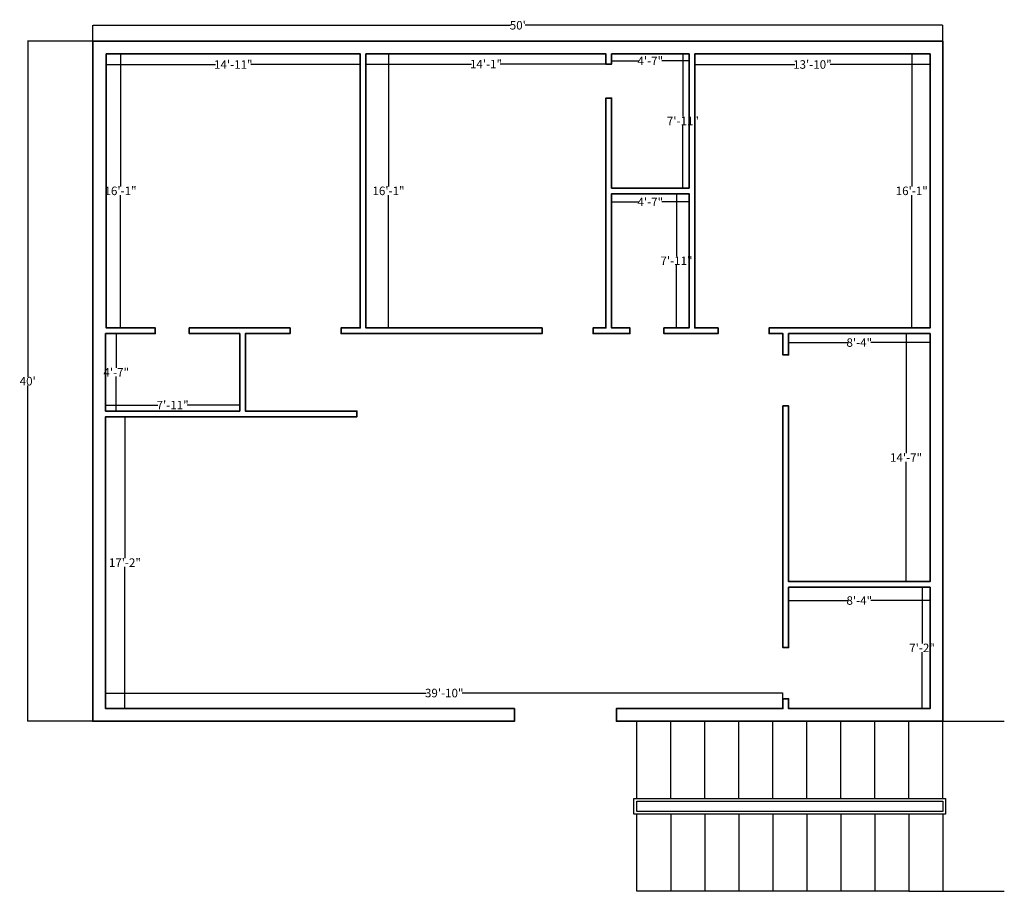
# Model space of a CAD drawing. Units: feet. Extents: x 3511 to 6270, y 2172 to 4127.
# Tile 2 of 4: x 4345 to 5040, y 3449 to 4064. Entities that reach past the tile are written whole.
import ezdxf

# ---------------------------------------------------------------- set-up
doc = ezdxf.new("R2010")
doc.units = ezdxf.units.FT
for name, color, linetype, lineweight in [('A-ANNO-DIMS', 2, 'Continuous', 18), ('A-FLOR-STRS', 4, 'Continuous', 25), ('A-WALL', 7, 'Continuous', 35)]:
    doc.layers.add(name, color=color, linetype=linetype, lineweight=lineweight)
doc.styles.get("Standard").update_dxf_attribs({"font": 'arial.ttf'})
doc.dimstyles.get("Standard").update_dxf_attribs({"dimtxt": 6, "dimasz": 0.18, "dimexe": 0.18, "dimexo": 0.0625, "dimgap": 0.09, "dimtad": 0, "dimtih": 1, "dimtoh": 1, "dimdec": 0, "dimzin": 0, "dimdsep": 46, "dimlunit": 3, "dimtxsty": 'Standard', "dimcen": 0.09, "dimadec": 0, "dimazin": 0, "dimtfac": 1, "dimtdec": 0, "dimtofl": 0, "dimtmove": 0, "dimatfit": 3, "dimfxl": 1, "dimtolj": 1, "dimtzin": 0, "dimarcsym": 0})

# ---------------------------------------------------------------- blocks, each defined once
blk = doc.blocks.new('*D32')
at = {"layer": 'A-ANNO-DIMS', "color": 0, "lineweight": -2, "transparency": 16777216}
for p, q in [((4405.77, 4039.51), (4405.77, 4031.86)), ((4585.11, 4039.51), (4585.11, 4031.86)), ((4405.95, 4032.04), (4483, 4032.04)), ((4584.93, 4032.04), (4507.88, 4032.04))]:
    blk.add_line(p, q, dxfattribs=at)
at = {"layer": 'A-ANNO-DIMS', "color": 0, "transparency": 16777216}
for points in [[(4405.95, 4032.07), (4405.95, 4032.01), (4405.77, 4032.04)], [(4584.93, 4032.07), (4584.93, 4032.01), (4585.11, 4032.04)]]:
    blk.add_solid(points, dxfattribs=at)
at = {"layer": 'Defpoints', "color": 0, "transparency": 16777216}
for p in [(4405.77, 4039.58), (4585.11, 4039.58), (4585.11, 4032.04)]:
    blk.add_point(p, dxfattribs=at)
at = {"layer": 'A-ANNO-DIMS', "color": 0, "transparency": 16777216, "insert": (4495.44, 4032.04), "char_height": 6, "attachment_point": 5}
blk.add_mtext('\\A1;14\'-11"', dxfattribs=at)
blk = doc.blocks.new('*D23')
at = {"layer": 'A-ANNO-DIMS', "color": 0, "lineweight": -2, "transparency": 16777216}
for p, q in [((4405.83, 4039.58), (4416.04, 4039.58)), ((4415.86, 4039.4), (4415.86, 3946.05)), ((4415.86, 3846.39), (4415.86, 3939.74)), ((4405.83, 3846.21), (4416.04, 3846.21))]:
    blk.add_line(p, q, dxfattribs=at)
at = {"layer": 'A-ANNO-DIMS', "color": 0, "transparency": 16777216}
for points in [[(4415.83, 4039.4), (4415.89, 4039.4), (4415.86, 4039.58)], [(4415.83, 3846.39), (4415.89, 3846.39), (4415.86, 3846.21)]]:
    blk.add_solid(points, dxfattribs=at)
at = {"layer": 'Defpoints', "color": 0, "transparency": 16777216}
for p in [(4405.77, 4039.58), (4405.77, 3846.21), (4415.86, 3846.21)]:
    blk.add_point(p, dxfattribs=at)
at = {"layer": 'A-ANNO-DIMS', "color": 0, "transparency": 16777216, "insert": (4415.86, 3942.89), "char_height": 6, "attachment_point": 5}
blk.add_mtext('\\A1;16\'-1"', dxfattribs=at)
blk = doc.blocks.new('*D24')
at = {"layer": 'A-ANNO-DIMS', "color": 0, "lineweight": -2, "transparency": 16777216}
for p, q in [((4589.11, 4039.51), (4589.11, 4032.14)), ((4758.44, 4039.51), (4758.44, 4032.14)), ((4589.29, 4032.32), (4663.66, 4032.32)), ((4758.26, 4032.32), (4683.89, 4032.32))]:
    blk.add_line(p, q, dxfattribs=at)
at = {"layer": 'A-ANNO-DIMS', "color": 0, "transparency": 16777216}
for points in [[(4589.29, 4032.35), (4589.29, 4032.29), (4589.11, 4032.32)], [(4758.26, 4032.35), (4758.26, 4032.29), (4758.44, 4032.32)]]:
    blk.add_solid(points, dxfattribs=at)
at = {"layer": 'Defpoints', "color": 0, "transparency": 16777216}
for p in [(4589.11, 4039.58), (4758.44, 4039.58), (4758.44, 4032.32)]:
    blk.add_point(p, dxfattribs=at)
at = {"layer": 'A-ANNO-DIMS', "color": 0, "transparency": 16777216, "insert": (4673.78, 4032.32), "char_height": 6, "attachment_point": 5}
blk.add_mtext('\\A1;14\'-1"', dxfattribs=at)
blk = doc.blocks.new('*D25')
at = {"layer": 'A-ANNO-DIMS', "color": 0, "lineweight": -2, "transparency": 16777216}
for p, q in [((4589.17, 4039.58), (4605.2, 4039.58)), ((4605.02, 4039.4), (4605.02, 3946.05)), ((4605.02, 3846.39), (4605.02, 3939.74)), ((4589.17, 3846.21), (4605.2, 3846.21))]:
    blk.add_line(p, q, dxfattribs=at)
at = {"layer": 'A-ANNO-DIMS', "color": 0, "transparency": 16777216}
for points in [[(4604.99, 4039.4), (4605.05, 4039.4), (4605.02, 4039.58)], [(4604.99, 3846.39), (4605.05, 3846.39), (4605.02, 3846.21)]]:
    blk.add_solid(points, dxfattribs=at)
at = {"layer": 'Defpoints', "color": 0, "transparency": 16777216}
for p in [(4589.11, 4039.58), (4589.11, 3846.21), (4605.02, 3846.21)]:
    blk.add_point(p, dxfattribs=at)
at = {"layer": 'A-ANNO-DIMS', "color": 0, "transparency": 16777216, "insert": (4605.02, 3942.89), "char_height": 6, "attachment_point": 5}
blk.add_mtext('\\A1;16\'-1"', dxfattribs=at)
blk = doc.blocks.new('*D26')
at = {"layer": 'A-ANNO-DIMS', "color": 0, "lineweight": -2, "transparency": 16777216}
for p, q in [((4762.44, 4039.51), (4762.44, 4034.45)), ((4817.15, 4039.51), (4817.15, 4034.45)), ((4762.62, 4034.63), (4781.61, 4034.63)), ((4816.97, 4034.63), (4797.98, 4034.63))]:
    blk.add_line(p, q, dxfattribs=at)
at = {"layer": 'A-ANNO-DIMS', "color": 0, "transparency": 16777216}
for points in [[(4762.62, 4034.66), (4762.62, 4034.6), (4762.44, 4034.63)], [(4816.97, 4034.66), (4816.97, 4034.6), (4817.15, 4034.63)]]:
    blk.add_solid(points, dxfattribs=at)
at = {"layer": 'Defpoints', "color": 0, "transparency": 16777216}
for p in [(4762.44, 4039.58), (4817.15, 4039.58), (4817.15, 4034.63)]:
    blk.add_point(p, dxfattribs=at)
at = {"layer": 'A-ANNO-DIMS', "color": 0, "transparency": 16777216, "insert": (4789.8, 4034.63), "char_height": 6, "attachment_point": 5}
blk.add_mtext('\\A1;4\'-7"', dxfattribs=at)
blk = doc.blocks.new('*D27')
at = {"layer": 'A-ANNO-DIMS', "color": 0, "lineweight": -2, "transparency": 16777216}
for p, q in [((4817.09, 4039.58), (4812.63, 4039.58)), ((4812.81, 4039.4), (4812.81, 3995.34)), ((4812.81, 3945.07), (4812.81, 3989.13)), ((4817.09, 3944.89), (4812.63, 3944.89))]:
    blk.add_line(p, q, dxfattribs=at)
at = {"layer": 'A-ANNO-DIMS', "color": 0, "transparency": 16777216}
for points in [[(4812.78, 4039.4), (4812.84, 4039.4), (4812.81, 4039.58)], [(4812.78, 3945.07), (4812.84, 3945.07), (4812.81, 3944.89)]]:
    blk.add_solid(points, dxfattribs=at)
at = {"layer": 'Defpoints', "color": 0, "transparency": 16777216}
for p in [(4817.15, 4039.58), (4812.81, 3944.89), (4817.15, 3944.89)]:
    blk.add_point(p, dxfattribs=at)
at = {"layer": 'A-ANNO-DIMS', "color": 0, "transparency": 16777216, "insert": (4812.81, 3992.23), "char_height": 6, "attachment_point": 5}
blk.add_mtext('\\A1;7\'-11"', dxfattribs=at)
blk = doc.blocks.new('*D28')
at = {"layer": 'A-ANNO-DIMS', "color": 0, "lineweight": -2, "transparency": 16777216}
for p, q in [((4821.15, 4039.51), (4821.15, 4031.89)), ((4987.28, 4039.51), (4987.28, 4031.89)), ((4821.33, 4032.07), (4891.77, 4032.07)), ((4987.1, 4032.07), (4916.66, 4032.07))]:
    blk.add_line(p, q, dxfattribs=at)
at = {"layer": 'A-ANNO-DIMS', "color": 0, "transparency": 16777216}
for points in [[(4821.33, 4032.1), (4821.33, 4032.04), (4821.15, 4032.07)], [(4987.1, 4032.1), (4987.1, 4032.04), (4987.28, 4032.07)]]:
    blk.add_solid(points, dxfattribs=at)
at = {"layer": 'Defpoints', "color": 0, "transparency": 16777216}
for p in [(4821.15, 4039.58), (4987.28, 4039.58), (4987.28, 4032.07)]:
    blk.add_point(p, dxfattribs=at)
at = {"layer": 'A-ANNO-DIMS', "color": 0, "transparency": 16777216, "insert": (4904.22, 4032.07), "char_height": 6, "attachment_point": 5}
blk.add_mtext('\\A1;13\'-10"', dxfattribs=at)
blk = doc.blocks.new('*D29')
at = {"layer": 'A-ANNO-DIMS', "color": 0, "lineweight": -2, "transparency": 16777216}
for p, q in [((4987.22, 4039.58), (4974.16, 4039.58)), ((4974.34, 4039.4), (4974.34, 3946.05)), ((4974.34, 3846.39), (4974.34, 3939.74)), ((4987.22, 3846.21), (4974.16, 3846.21))]:
    blk.add_line(p, q, dxfattribs=at)
at = {"layer": 'A-ANNO-DIMS', "color": 0, "transparency": 16777216}
for points in [[(4974.31, 4039.4), (4974.37, 4039.4), (4974.34, 4039.58)], [(4974.31, 3846.39), (4974.37, 3846.39), (4974.34, 3846.21)]]:
    blk.add_solid(points, dxfattribs=at)
at = {"layer": 'Defpoints', "color": 0, "transparency": 16777216}
for p in [(4987.28, 4039.58), (4974.34, 3846.21), (4987.28, 3846.21)]:
    blk.add_point(p, dxfattribs=at)
at = {"layer": 'A-ANNO-DIMS', "color": 0, "transparency": 16777216, "insert": (4974.34, 3942.89), "char_height": 6, "attachment_point": 5}
blk.add_mtext('\\A1;16\'-1"', dxfattribs=at)
blk = doc.blocks.new('*D30')
at = {"layer": 'A-ANNO-DIMS', "color": 0, "lineweight": -2, "transparency": 16777216}
for p, q in [((4817.09, 3940.89), (4808.08, 3940.89)), ((4808.26, 3940.71), (4808.26, 3896.65)), ((4808.26, 3846.39), (4808.26, 3890.45)), ((4817.09, 3846.21), (4808.08, 3846.21))]:
    blk.add_line(p, q, dxfattribs=at)
at = {"layer": 'A-ANNO-DIMS', "color": 0, "transparency": 16777216}
for points in [[(4808.23, 3940.71), (4808.29, 3940.71), (4808.26, 3940.89)], [(4808.23, 3846.39), (4808.29, 3846.39), (4808.26, 3846.21)]]:
    blk.add_solid(points, dxfattribs=at)
at = {"layer": 'Defpoints', "color": 0, "transparency": 16777216}
for p in [(4817.15, 3940.89), (4808.26, 3846.21), (4817.15, 3846.21)]:
    blk.add_point(p, dxfattribs=at)
at = {"layer": 'A-ANNO-DIMS', "color": 0, "transparency": 16777216, "insert": (4808.26, 3893.55), "char_height": 6, "attachment_point": 5}
blk.add_mtext('\\A1;7\'-11"', dxfattribs=at)
blk = doc.blocks.new('*D31')
at = {"layer": 'A-ANNO-DIMS', "color": 0, "lineweight": -2, "transparency": 16777216}
for p, q in [((4762.44, 3940.83), (4762.44, 3934.92)), ((4817.15, 3940.83), (4817.15, 3934.92)), ((4762.62, 3935.1), (4781.61, 3935.1)), ((4816.97, 3935.1), (4797.98, 3935.1))]:
    blk.add_line(p, q, dxfattribs=at)
at = {"layer": 'A-ANNO-DIMS', "color": 0, "transparency": 16777216}
for points in [[(4762.62, 3935.13), (4762.62, 3935.07), (4762.44, 3935.1)], [(4816.97, 3935.13), (4816.97, 3935.07), (4817.15, 3935.1)]]:
    blk.add_solid(points, dxfattribs=at)
at = {"layer": 'Defpoints', "color": 0, "transparency": 16777216}
for p in [(4762.44, 3940.89), (4817.15, 3940.89), (4817.15, 3935.1)]:
    blk.add_point(p, dxfattribs=at)
at = {"layer": 'A-ANNO-DIMS', "color": 0, "transparency": 16777216, "insert": (4789.8, 3935.1), "char_height": 6, "attachment_point": 5}
blk.add_mtext('\\A1;4\'-7"', dxfattribs=at)
blk = doc.blocks.new('*D33')
at = {"layer": 'A-ANNO-DIMS', "color": 0, "lineweight": -2, "transparency": 16777216}
for p, q in [((4405.28, 3787.57), (4405.28, 3791.87)), ((4405.46, 3791.69), (4442.25, 3791.69)), ((4499.79, 3791.69), (4462.99, 3791.69)), ((4499.97, 3787.57), (4499.97, 3791.87))]:
    blk.add_line(p, q, dxfattribs=at)
at = {"layer": 'A-ANNO-DIMS', "color": 0, "transparency": 16777216}
for points in [[(4405.46, 3791.72), (4405.46, 3791.66), (4405.28, 3791.69)], [(4499.79, 3791.72), (4499.79, 3791.66), (4499.97, 3791.69)]]:
    blk.add_solid(points, dxfattribs=at)
at = {"layer": 'Defpoints', "color": 0, "transparency": 16777216}
for p in [(4499.97, 3791.69), (4405.28, 3787.5), (4499.97, 3787.5)]:
    blk.add_point(p, dxfattribs=at)
at = {"layer": 'A-ANNO-DIMS', "color": 0, "transparency": 16777216, "insert": (4452.62, 3791.69), "char_height": 6, "attachment_point": 5}
blk.add_mtext('\\A1;7\'-11"', dxfattribs=at)
blk = doc.blocks.new('*D34')
at = {"layer": 'A-ANNO-DIMS', "color": 0, "lineweight": -2, "transparency": 16777216}
for p, q in [((4405.34, 3842.21), (4412.98, 3842.21)), ((4412.8, 3842.03), (4412.8, 3817.95)), ((4412.8, 3787.68), (4412.8, 3811.77)), ((4405.34, 3787.5), (4412.98, 3787.5))]:
    blk.add_line(p, q, dxfattribs=at)
at = {"layer": 'A-ANNO-DIMS', "color": 0, "transparency": 16777216}
for points in [[(4412.77, 3842.03), (4412.83, 3842.03), (4412.8, 3842.21)], [(4412.77, 3787.68), (4412.83, 3787.68), (4412.8, 3787.5)]]:
    blk.add_solid(points, dxfattribs=at)
at = {"layer": 'Defpoints', "color": 0, "transparency": 16777216}
for p in [(4405.28, 3842.21), (4412.8, 3842.21), (4405.28, 3787.5)]:
    blk.add_point(p, dxfattribs=at)
at = {"layer": 'A-ANNO-DIMS', "color": 0, "transparency": 16777216, "insert": (4412.8, 3814.86), "char_height": 6, "attachment_point": 5}
blk.add_mtext('\\A1;4\'-7"', dxfattribs=at)
blk = doc.blocks.new('*D35')
at = {"layer": 'A-ANNO-DIMS', "color": 0, "lineweight": -2, "transparency": 16777216}
for p, q in [((4405.28, 3577.64), (4405.28, 3588.67)), ((4405.46, 3588.49), (4631.6, 3588.49)), ((4883.19, 3588.49), (4657.05, 3588.49)), ((4883.37, 3577.64), (4883.37, 3588.67))]:
    blk.add_line(p, q, dxfattribs=at)
at = {"layer": 'A-ANNO-DIMS', "color": 0, "transparency": 16777216}
for points in [[(4405.46, 3588.52), (4405.46, 3588.46), (4405.28, 3588.49)], [(4883.19, 3588.52), (4883.19, 3588.46), (4883.37, 3588.49)]]:
    blk.add_solid(points, dxfattribs=at)
at = {"layer": 'Defpoints', "color": 0, "transparency": 16777216}
for p in [(4883.37, 3588.49), (4405.28, 3577.58), (4883.37, 3577.58)]:
    blk.add_point(p, dxfattribs=at)
at = {"layer": 'A-ANNO-DIMS', "color": 0, "transparency": 16777216, "insert": (4644.33, 3588.49), "char_height": 6, "attachment_point": 5}
blk.add_mtext('\\A1;39\'-10"', dxfattribs=at)
blk = doc.blocks.new('*D36')
at = {"layer": 'A-ANNO-DIMS', "color": 0, "lineweight": -2, "transparency": 16777216}
for p, q in [((4405.34, 3783.5), (4419.1, 3783.5)), ((4418.92, 3783.32), (4418.92, 3683.64)), ((4418.92, 3577.76), (4418.92, 3677.44)), ((4405.34, 3577.58), (4419.1, 3577.58))]:
    blk.add_line(p, q, dxfattribs=at)
at = {"layer": 'A-ANNO-DIMS', "color": 0, "transparency": 16777216}
for points in [[(4418.89, 3783.32), (4418.95, 3783.32), (4418.92, 3783.5)], [(4418.89, 3577.76), (4418.95, 3577.76), (4418.92, 3577.58)]]:
    blk.add_solid(points, dxfattribs=at)
at = {"layer": 'Defpoints', "color": 0, "transparency": 16777216}
for p in [(4405.28, 3783.5), (4405.28, 3577.58), (4418.92, 3577.58)]:
    blk.add_point(p, dxfattribs=at)
at = {"layer": 'A-ANNO-DIMS', "color": 0, "transparency": 16777216, "insert": (4418.92, 3680.54), "char_height": 6, "attachment_point": 5}
blk.add_mtext('\\A1;17\'-2"', dxfattribs=at)
blk = doc.blocks.new('*D37')
at = {"layer": 'A-ANNO-DIMS', "color": 0, "lineweight": -2, "transparency": 16777216}
for p, q in [((4987.22, 3842.21), (4970.13, 3842.21)), ((4970.31, 3842.03), (4970.31, 3757.78)), ((4970.31, 3667.33), (4970.31, 3751.57)), ((4987.22, 3667.15), (4970.13, 3667.15))]:
    blk.add_line(p, q, dxfattribs=at)
at = {"layer": 'A-ANNO-DIMS', "color": 0, "transparency": 16777216}
for points in [[(4970.28, 3842.03), (4970.34, 3842.03), (4970.31, 3842.21)], [(4970.28, 3667.33), (4970.34, 3667.33), (4970.31, 3667.15)]]:
    blk.add_solid(points, dxfattribs=at)
at = {"layer": 'Defpoints', "color": 0, "transparency": 16777216}
for p in [(4987.28, 3842.21), (4970.31, 3667.15), (4987.28, 3667.15)]:
    blk.add_point(p, dxfattribs=at)
at = {"layer": 'A-ANNO-DIMS', "color": 0, "transparency": 16777216, "insert": (4970.31, 3754.68), "char_height": 6, "attachment_point": 5}
blk.add_mtext('\\A1;14\'-7"', dxfattribs=at)
blk = doc.blocks.new('*D38')
at = {"layer": 'A-ANNO-DIMS', "color": 0, "lineweight": -2, "transparency": 16777216}
for p, q in [((4887.37, 3842.15), (4887.37, 3835.65)), ((4987.28, 3842.15), (4987.28, 3835.65)), ((4887.55, 3835.83), (4929.26, 3835.83)), ((4987.1, 3835.83), (4945.39, 3835.83))]:
    blk.add_line(p, q, dxfattribs=at)
at = {"layer": 'A-ANNO-DIMS', "color": 0, "transparency": 16777216}
for points in [[(4887.55, 3835.86), (4887.55, 3835.8), (4887.37, 3835.83)], [(4987.1, 3835.86), (4987.1, 3835.8), (4987.28, 3835.83)]]:
    blk.add_solid(points, dxfattribs=at)
at = {"layer": 'Defpoints', "color": 0, "transparency": 16777216}
for p in [(4887.37, 3842.21), (4987.28, 3842.21), (4887.37, 3835.83)]:
    blk.add_point(p, dxfattribs=at)
at = {"layer": 'A-ANNO-DIMS', "color": 0, "transparency": 16777216, "insert": (4937.33, 3835.83), "char_height": 6, "attachment_point": 5}
blk.add_mtext('\\A1;8\'-4"', dxfattribs=at)
blk = doc.blocks.new('*D39')
at = {"layer": 'A-ANNO-DIMS', "color": 0, "lineweight": -2, "transparency": 16777216}
for p, q in [((4987.22, 3663.15), (4981.44, 3663.15)), ((4981.62, 3662.97), (4981.62, 3623.46)), ((4981.62, 3577.76), (4981.62, 3617.26)), ((4987.22, 3577.58), (4981.44, 3577.58))]:
    blk.add_line(p, q, dxfattribs=at)
at = {"layer": 'A-ANNO-DIMS', "color": 0, "transparency": 16777216}
for points in [[(4981.59, 3662.97), (4981.65, 3662.97), (4981.62, 3663.15)], [(4981.59, 3577.76), (4981.65, 3577.76), (4981.62, 3577.58)]]:
    blk.add_solid(points, dxfattribs=at)
at = {"layer": 'Defpoints', "color": 0, "transparency": 16777216}
for p in [(4987.28, 3663.15), (4981.62, 3577.58), (4987.28, 3577.58)]:
    blk.add_point(p, dxfattribs=at)
at = {"layer": 'A-ANNO-DIMS', "color": 0, "transparency": 16777216, "insert": (4981.62, 3620.36), "char_height": 6, "attachment_point": 5}
blk.add_mtext('\\A1;7\'-2"', dxfattribs=at)
blk = doc.blocks.new('*D40')
at = {"layer": 'A-ANNO-DIMS', "color": 0, "lineweight": -2, "transparency": 16777216}
for p, q in [((4887.37, 3663.08), (4887.37, 3653.6)), ((4987.28, 3663.08), (4987.28, 3653.6)), ((4887.55, 3653.78), (4929.26, 3653.78)), ((4987.1, 3653.78), (4945.39, 3653.78))]:
    blk.add_line(p, q, dxfattribs=at)
at = {"layer": 'A-ANNO-DIMS', "color": 0, "transparency": 16777216}
for points in [[(4887.55, 3653.81), (4887.55, 3653.75), (4887.37, 3653.78)], [(4987.1, 3653.81), (4987.1, 3653.75), (4987.28, 3653.78)]]:
    blk.add_solid(points, dxfattribs=at)
at = {"layer": 'Defpoints', "color": 0, "transparency": 16777216}
for p in [(4887.37, 3663.15), (4987.28, 3663.15), (4887.37, 3653.78)]:
    blk.add_point(p, dxfattribs=at)
at = {"layer": 'A-ANNO-DIMS', "color": 0, "transparency": 16777216, "insert": (4937.33, 3653.78), "char_height": 6, "attachment_point": 5}
blk.add_mtext('\\A1;8\'-4"', dxfattribs=at)
blk = doc.blocks.new('*D41')
at = {"layer": 'A-ANNO-DIMS', "color": 0, "lineweight": -2, "transparency": 16777216}
for p, q in [((4396.22, 4048.58), (4350.17, 4048.58)), ((4350.35, 4048.4), (4350.35, 3811.73)), ((4350.35, 3568.76), (4350.35, 3805.42)), ((4396.22, 3568.58), (4350.17, 3568.58))]:
    blk.add_line(p, q, dxfattribs=at)
at = {"layer": 'A-ANNO-DIMS', "color": 0, "transparency": 16777216}
for points in [[(4350.32, 4048.4), (4350.38, 4048.4), (4350.35, 4048.58)], [(4350.32, 3568.76), (4350.38, 3568.76), (4350.35, 3568.58)]]:
    blk.add_solid(points, dxfattribs=at)
at = {"layer": 'Defpoints', "color": 0, "transparency": 16777216}
for p in [(4396.28, 4048.58), (4350.35, 3568.58), (4396.28, 3568.58)]:
    blk.add_point(p, dxfattribs=at)
at = {"layer": 'A-ANNO-DIMS', "color": 0, "transparency": 16777216, "insert": (4350.35, 3808.58), "char_height": 6, "attachment_point": 5}
blk.add_mtext("\\A1;40'", dxfattribs=at)
blk = doc.blocks.new('*D42')
at = {"layer": 'A-ANNO-DIMS', "color": 0, "lineweight": -2, "transparency": 16777216}
for p, q in [((4396.28, 4048.64), (4396.28, 4059.92)), ((4396.46, 4059.74), (4691.1, 4059.74)), ((4996.1, 4059.74), (4701.46, 4059.74)), ((4996.28, 4048.64), (4996.28, 4059.92))]:
    blk.add_line(p, q, dxfattribs=at)
at = {"layer": 'A-ANNO-DIMS', "color": 0, "transparency": 16777216}
for points in [[(4396.46, 4059.77), (4396.46, 4059.71), (4396.28, 4059.74)], [(4996.1, 4059.77), (4996.1, 4059.71), (4996.28, 4059.74)]]:
    blk.add_solid(points, dxfattribs=at)
at = {"layer": 'Defpoints', "color": 0, "transparency": 16777216}
for p in [(4996.28, 4059.74), (4396.28, 4048.58), (4996.28, 4048.58)]:
    blk.add_point(p, dxfattribs=at)
at = {"layer": 'A-ANNO-DIMS', "color": 0, "transparency": 16777216, "insert": (4696.28, 4059.74), "char_height": 6, "attachment_point": 5}
blk.add_mtext("\\A1;50'", dxfattribs=at)
blk = doc.blocks.new('STAIR')
for p, q in [((2, 65.57), (2, 120)), ((26, 65.57), (26, 120)), ((50, 65.57), (50, 120)), ((74, 65.57), (74, 120)), ((98, 65.57), (98, 120)), ((122, 65.57), (122, 120)), ((146, 65.57), (146, 120)), ((170, 65.57), (170, 120)), ((194, 65.57), (194, 120)), ((218, 54.42), (218, 0))]:
    blk.add_line(p, q)
for points in [[(218, 65.57), (218, 120), (261.4, 120)], [(26, 54.42), (26, 0), (14, 0), (2, 0), (2, 54.42)], [(50, 54.42), (50, 0), (38, 0), (26, 0)], [(74, 54.42), (74, 0), (62, 0), (50, 0)], [(98, 54.42), (98, 0), (86, 0), (74, 0)], [(122, 54.42), (122, 0), (110, 0), (98, 0)], [(146, 54.42), (146, 0), (134, 0), (122, 0)], [(170, 54.42), (170, 0), (158, 0), (146, 0)], [(194, 54.42), (194, 0), (182, 0), (170, 0)], [(194, 0), (206, 0), (218, 0), (261.4, 0)]]:
    blk.add_lwpolyline(points)
for points in [[(0, 65.57), (220, 65.57), (220, 54.42), (0, 54.42)], [(218, 56.42), (2, 56.42), (2, 63.57), (218, 63.57)]]:
    blk.add_lwpolyline(points, close=True)

msp = doc.modelspace()

# ---------------------------------------------------------------- linework, layer by layer
at = {"layer": 'A-WALL'}
msp.add_lwpolyline([(4887.37, 3663.15), (4887.37, 3620.52), (4883.37, 3620.52), (4883.37, 3791.14), (4887.37, 3791.14), (4887.37, 3667.15), (4987.28, 3667.15), (4987.28, 3842.21), (4887.37, 3842.21), (4887.37, 3827.14), (4883.37, 3827.14), (4883.37, 3842.21), (4873.69, 3842.21), (4873.69, 3846.21), (4987.28, 3846.21), (4987.28, 4039.58), (4821.15, 4039.58), (4821.15, 3846.21), (4837.69, 3846.21), (4837.69, 3842.21), (4799.38, 3842.21), (4799.38, 3846.21), (4817.15, 3846.21), (4817.15, 3940.89), (4762.44, 3940.89), (4762.44, 3846.21), (4775.38, 3846.21), (4775.38, 3842.21), (4749.44, 3842.21), (4749.44, 3846.21), (4758.44, 3846.21), (4758.44, 4008.32), (4762.44, 4008.32), (4762.44, 3944.89), (4817.15, 3944.89), (4817.15, 4039.58), (4762.44, 4039.58), (4762.44, 4032.32), (4758.44, 4032.32), (4758.44, 4039.58), (4589.11, 4039.58), (4589.11, 3846.21), (4713.44, 3846.21), (4713.44, 3842.21), (4571.55, 3842.21), (4571.55, 3846.21), (4585.11, 3846.21), (4585.11, 4039.58), (4405.77, 4039.58), (4405.77, 3846.21), (4440.3, 3846.21), (4440.3, 3842.21), (4405.28, 3842.21), (4405.28, 3787.5), (4405.28, 3787.5), (4499.97, 3787.5), (4499.97, 3842.21), (4464.3, 3842.21), (4464.3, 3846.21), (4535.55, 3846.21), (4535.55, 3842.21), (4503.97, 3842.21), (4503.97, 3787.51), (4582.72, 3787.51), (4582.72, 3783.5), (4405.28, 3783.5), (4405.28, 3577.58), (4693.92, 3577.58), (4693.92, 3568.58), (4396.28, 3568.58), (4396.28, 4048.58), (4996.28, 4048.58), (4996.28, 3568.58), (4765.92, 3568.58), (4765.92, 3577.58), (4883.37, 3577.58), (4883.37, 3584.52), (4887.37, 3584.52), (4887.37, 3577.58), (4987.28, 3577.58), (4987.28, 3663.15)], close=True, dxfattribs=at)
msp.add_lwpolyline([(4503.97, 3783.5), (4503.97, 3783.5)], dxfattribs=at)

# ---------------------------------------------------------------- block references
at = {"layer": 'A-FLOR-STRS'}
msp.add_blockref('STAIR', (4778.28, 3448.58), dxfattribs=at)

# ---------------------------------------------------------------- dimensions: what is measured, and where the dimension line sits
at = {"layer": 'A-ANNO-DIMS'}
for base, p1, p2, picture, middle in [((4996.28, 4059.74), (4396.28, 4048.58), (4996.28, 4048.58), '*D42', (4696.28, 4059.74)), ((4585.11, 4032.04), (4405.77, 4039.58), (4585.11, 4039.58), '*D32', (4495.44, 4032.04)), ((4758.44, 4032.32), (4589.11, 4039.58), (4758.44, 4039.58), '*D24', (4673.78, 4032.32)), ((4817.15, 4034.63), (4762.44, 4039.58), (4817.15, 4039.58), '*D26', (4789.8, 4034.63)), ((4987.28, 4032.07), (4821.15, 4039.58), (4987.28, 4039.58), '*D28', (4904.22, 4032.07)), ((4817.15, 3935.1), (4762.44, 3940.89), (4817.15, 3940.89), '*D31', (4789.8, 3935.1)), ((4887.37, 3835.83), (4987.28, 3842.21), (4887.37, 3842.21), '*D38', (4937.33, 3835.83)), ((4499.97, 3791.69), (4405.28, 3787.5), (4499.97, 3787.5), '*D33', (4452.62, 3791.69)), ((4887.37, 3653.78), (4987.28, 3663.15), (4887.37, 3663.15), '*D40', (4937.33, 3653.78)), ((4883.37, 3588.49), (4405.28, 3577.58), (4883.37, 3577.58), '*D35', (4644.33, 3588.49))]:
    dim = msp.add_linear_dim(base=base, p1=p1, p2=p2, dimstyle='Standard', override={"dimclrd": 0, "dimclre": 0, "dimclrt": 0}, dxfattribs=at)
    dim.commit()
    dim.dimension.update_dxf_attribs({"geometry": picture, "text_midpoint": middle})
for base, p1, p2, picture, middle in [((4350.35, 3568.58), (4396.28, 4048.58), (4396.28, 3568.58), '*D41', (4350.35, 3808.58)), ((4415.86, 3846.21), (4405.77, 4039.58), (4405.77, 3846.21), '*D23', (4415.86, 3942.89)), ((4605.02, 3846.21), (4589.11, 4039.58), (4589.11, 3846.21), '*D25', (4605.02, 3942.89)), ((4812.81, 3944.89), (4817.15, 4039.58), (4817.15, 3944.89), '*D27', (4812.81, 3992.23)), ((4974.34, 3846.21), (4987.28, 4039.58), (4987.28, 3846.21), '*D29', (4974.34, 3942.89)), ((4808.26, 3846.21), (4817.15, 3940.89), (4817.15, 3846.21), '*D30', (4808.26, 3893.55)), ((4412.8, 3842.21), (4405.28, 3787.5), (4405.28, 3842.21), '*D34', (4412.8, 3814.86)), ((4970.31, 3667.15), (4987.28, 3842.21), (4987.28, 3667.15), '*D37', (4970.31, 3754.68)), ((4418.92, 3577.58), (4405.28, 3783.5), (4405.28, 3577.58), '*D36', (4418.92, 3680.54)), ((4981.62, 3577.58), (4987.28, 3663.15), (4987.28, 3577.58), '*D39', (4981.62, 3620.36))]:
    dim = msp.add_linear_dim(base=base, p1=p1, p2=p2, angle=90, dimstyle='Standard', override={"dimclrd": 0, "dimclre": 0, "dimclrt": 0}, dxfattribs=at)
    dim.commit()
    dim.dimension.update_dxf_attribs({"geometry": picture, "text_midpoint": middle})

doc.saveas('drawing.dxf')
